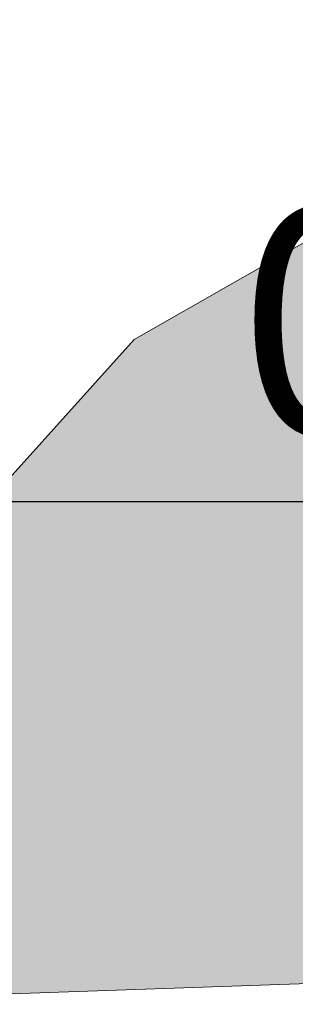
# Model space of a CAD drawing. Units: inches. Extents: x 2091 to 2899, y 967 to 2217.
# Tile 251 of 256: x 2217.01 to 2221.88, y 1131.25 to 1148.63. Entities that reach past the tile are written whole.
import ezdxf

# ---------------------------------------------------------------- set-up
doc = ezdxf.new("R2010")
doc.units = ezdxf.units.IN
doc.layers.add('A-ANNO-DIMS', color=2, linetype='Continuous', lineweight=18)
doc.layers.add('L-PLNT-TREE', color=94, linetype='Continuous', lineweight=13)
doc.layers.add('A-WALL-PATT', color=141, linetype='Continuous', lineweight=13, true_color=0xadddf7)
doc.layers.add('L-PLNT-PATT', color=114, linetype='Continuous', lineweight=13, true_color=0x139b48)
doc.styles.get("Standard").update_dxf_attribs({"font": 'arial.ttf'})
doc.dimstyles.new('ISO-25', dxfattribs={"dimtxt": 4, "dimasz": 4, "dimexe": 1.25, "dimexo": 0.625, "dimtad": 1, "dimdec": 0, "dimlunit": 3, "dimtxsty": 'Standard', "dimcen": 2.5, "dimadec": 0, "dimazin": 0, "dimtfac": 1, "dimtdec": 0, "dimtmove": 0, "dimatfit": 3, "dimfxl": 1, "dimarcsym": 0})

# ---------------------------------------------------------------- blocks, each defined once
blk = doc.blocks.new('*U25')
blk.add_lwpolyline([(-1139.42368, 1783.79628), (-1216.11644, 1685.47796), (-1117.5111, 1601.2033), (-1051.7759, 1643.3419), (-1126.09884, 1521.20092), (-1072.10606, 1527.49758), (-1079.90386, 1416.93646), (-1259.93906, 1179.83508), (-1479.05978, 1165.78888), (-1577.66258, 1109.60662), (-1742.00312, 927.01364), (-1676.26538, 814.64658), (-1270.89408, 828.69278), (-1194.20386, 772.51052), (-1007.95074, 856.78518), (-876.4778, 575.87134), (-821.70016, 575.87134), (-569.71184, 884.87504)])
blk = doc.blocks.new('*D37')
at = {"layer": 'A-ANNO-DIMS', "color": 0, "lineweight": -2, "transparency": 16777216}
for p, q in [((2203.116, 1151.622), (2203.116, 1138.874)), ((2212.276, 1151.622), (2212.276, 1138.874)), ((2199.116, 1140.124), (2195.116, 1140.124)), ((2203.116, 1140.124), (2212.276, 1140.124)), ((2216.276, 1140.124), (2245.908, 1140.124))]:
    blk.add_line(p, q, dxfattribs=at)
at = {"layer": 'A-ANNO-DIMS', "color": 0, "transparency": 16777216}
for points in [[(2199.116, 1140.79), (2199.116, 1139.457), (2203.116, 1140.124)], [(2216.276, 1140.79), (2216.276, 1139.457), (2212.276, 1140.124)]]:
    blk.add_solid(points, dxfattribs=at)
at = {"layer": 'Defpoints', "color": 0, "transparency": 16777216}
for p in [(2203.116, 1152.247), (2212.276, 1152.247), (2212.276, 1140.124)]:
    blk.add_point(p, dxfattribs=at)
at = {"layer": 'A-ANNO-DIMS', "color": 0, "transparency": 16777216, "insert": (2233.092, 1142.791), "char_height": 4, "attachment_point": 5}
blk.add_mtext('0\'-9" TYP.', dxfattribs=at)
blk = doc.blocks.new('*D71')
at = {"layer": 'A-ANNO-DIMS', "color": 0, "lineweight": -2, "transparency": 16777216}
for p, q in [((2212.144, 1351.294), (2212.144, 969.464)), ((2452.144, 1351.294), (2452.144, 969.464)), ((2216.144, 970.714), (2448.144, 970.714))]:
    blk.add_line(p, q, dxfattribs=at)
at = {"layer": 'A-ANNO-DIMS', "color": 0, "transparency": 16777216}
for points in [[(2216.144, 971.381), (2216.144, 970.048), (2212.144, 970.714)], [(2448.144, 971.381), (2448.144, 970.048), (2452.144, 970.714)]]:
    blk.add_solid(points, dxfattribs=at)
at = {"layer": 'Defpoints', "color": 0, "transparency": 16777216}
for p in [(2212.144, 1351.919), (2452.144, 1351.919), (2452.144, 970.714)]:
    blk.add_point(p, dxfattribs=at)
at = {"layer": 'A-ANNO-DIMS', "color": 0, "transparency": 16777216, "insert": (2332.144, 973.382), "char_height": 4, "attachment_point": 5}
blk.add_mtext('20\'-0"', dxfattribs=at)
blk = doc.blocks.new('*D75')
at = {"layer": 'A-ANNO-DIMS', "color": 0, "lineweight": -2, "transparency": 16777216}
for p, q in [((2212.144, 1274.794), (2212.144, 969.464)), ((2308.144, 1274.794), (2308.144, 969.464)), ((2216.144, 970.714), (2304.144, 970.714))]:
    blk.add_line(p, q, dxfattribs=at)
at = {"layer": 'A-ANNO-DIMS', "color": 0, "transparency": 16777216}
for points in [[(2216.144, 971.381), (2216.144, 970.048), (2212.144, 970.714)], [(2304.144, 971.381), (2304.144, 970.048), (2308.144, 970.714)]]:
    blk.add_solid(points, dxfattribs=at)
at = {"layer": 'Defpoints', "color": 0, "transparency": 16777216}
for p in [(2212.144, 1275.419), (2308.144, 1275.419), (2308.144, 970.714)]:
    blk.add_point(p, dxfattribs=at)
at = {"layer": 'A-ANNO-DIMS', "color": 0, "transparency": 16777216, "insert": (2260.144, 973.382), "char_height": 4, "attachment_point": 5}
blk.add_mtext('8\'-0"', dxfattribs=at)

msp = doc.modelspace()

# ---------------------------------------------------------------- hatches: boundary and pattern name
at = {"layer": 'A-WALL-PATT'}
h = msp.add_hatch(color=256, dxfattribs=at)
h.dxf.hatch_style = 1
h.paths.add_polyline_path([(2803.144, 2050.919), (2203.144, 2050.919), (2203.144, 1090.919), (2803.144, 1090.919)])
h.paths.add_polyline_path([(2635.799, 1147.54), (2674.524, 1147.54, 0.376086), (2678.53, 1152.88), (2678.53, 1159.556, 0.333335), (2674.524, 1163.562), (2674.524, 1163.562), (2674.524, 1192.934), (2635.806, 1192.934), (2597.088, 1192.934), (2597.088, 1163.562, 0.333335), (2593.082, 1159.556), (2593.082, 1152.88, 0.376086), (2597.088, 1147.54)], flags=0)
h.paths.add_polyline_path([(2436.01, 1278.241, 0.000483), (2435.953, 1278.215, -0.001328), (2435.936, 1278.112, -0.001711), (2436.116, 1278.041, 0.002185)], flags=0)
h.paths.add_polyline_path([(2794.144, 1143.419), (2794.144, 1347.419), (2543.37, 1347.419), (2543.37, 1351.919), (2794.144, 1351.919), (2794.144, 1392.714), (2793.947, 1392.714), (2793.947, 1473.537), (2794.144, 1473.537), (2794.144, 1531.919), (2650.144, 1531.919), (2650.144, 1536.419), (2794.144, 1536.419), (2794.144, 1692.419), (2609.376, 1692.419), (2609.376, 1644.419), (2604.876, 1644.419), (2604.876, 1744.919), (2609.376, 1744.919), (2609.376, 1696.919), (2794.144, 1696.919), (2794.144, 1780.919), (2609.644, 1780.919), (2493.876, 1780.919), (2493.876, 1785.419), (2609.644, 1785.419), (2794.144, 1785.419), (2794.144, 1847.939), (2793.951, 1847.939), (2793.951, 1928.762), (2794.144, 1928.762), (2794.144, 1941.419), (2614.144, 1941.419), (2614.144, 1821.419), (2609.644, 1821.419), (2609.644, 1941.419), (2392.144, 1941.419), (2392.144, 1819.919), (2387.644, 1819.919), (2387.644, 1941.419), (2212.144, 1941.419), (2212.144, 1783.919), (2392.144, 1783.919), (2392.144, 1780.919), (2212.144, 1780.919), (2212.144, 1629.419), (2387.644, 1629.419), (2387.644, 1744.919), (2392.144, 1744.919), (2392.144, 1627.919), (2317.144, 1627.919), (2317.144, 1551.419), (2317.144, 1536.419), (2459.384, 1536.419), (2459.384, 1602.396), (2463.884, 1602.396), (2463.884, 1531.919), (2456.644, 1531.919), (2456.644, 1529.919), (2452.144, 1529.919), (2452.144, 1531.919), (2312.644, 1531.919), (2312.644, 1551.419), (2306.144, 1551.419), (2306.144, 1555.919), (2308.144, 1555.919), (2308.144, 1551.419), (2312.644, 1551.419), (2312.644, 1627.919), (2212.144, 1627.919), (2212.144, 1555.919), (2270.144, 1555.919), (2270.144, 1551.419), (2212.144, 1551.419), (2212.144, 1351.919), (2272.144, 1351.919), (2272.144, 1347.419), (2212.144, 1347.419), (2212.144, 1275.419), (2308.144, 1275.419), (2308.144, 1351.919), (2452.144, 1351.919), (2452.144, 1493.919), (2456.644, 1493.919), (2456.644, 1347.419), (2312.644, 1347.419), (2312.644, 1270.919), (2212.144, 1270.919), (2212.144, 1099.919), (2281.238, 1099.919), (2282.871, 1110.914), (2282.008, 1116.997), (2278.558, 1121.42), (2268.206, 1128.056), (2272.088, 1128.056), (2273.813, 1131.927), (2279.42, 1134.692), (2285.028, 1135.245), (2287.616, 1137.457), (2288.047, 1138.01), (2289.341, 1140.775), (2291.067, 1139.669), (2292.361, 1135.245), (2295.38, 1136.904), (2296.243, 1135.798), (2297.105, 1133.033), (2300.125, 1138.01), (2303.144, 1138.01), (2304.438, 1135.798), (2303.144, 1133.586), (2306.595, 1134.692), (2307.889, 1133.033), (2310.908, 1135.245), (2313.927, 1134.139), (2315.627, 1132.427), (2308.32, 1117.55), (2290.204, 1109.808), (2288.91, 1103.172), (2289.272, 1099.919), (2434.918, 1099.919), (2431.593, 1124.788), (2429.93, 1169.553), (2430.927, 1240.52), (2435.659, 1238.186), (2437.135, 1196.554), (2438.798, 1143.973), (2442.678, 1111.998), (2446.558, 1099.919), (2794.144, 1099.919), (2794.144, 1138.919), (2548.032, 1138.919), (2548.032, 1143.419), (2548.032, 1148.819), (2546.668, 1148.032), (2528.686, 1179.179, 0.256256), (2512.032, 1148.819), (2512.032, 1143.419), (2512.032, 1138.919), (2507.532, 1138.919), (2507.532, 1143.419), (2507.532, 1148.819, 0.256256), (2490.879, 1179.179), (2472.896, 1148.032), (2471.532, 1148.819), (2471.532, 1143.419), (2467.032, 1143.419), (2467.032, 1269.946, 0.039061), (2460.91, 1273.58), (2467.032, 1273.58), (2467.032, 1286.325, 0.014511), (2465.216, 1286.762), (2467.032, 1287.053), (2467.032, 1323.419), (2471.532, 1323.419), (2471.532, 1148.819), (2489.532, 1179.996), (2490.896, 1179.208), (2490.879, 1179.179, -0.256256), (2507.532, 1148.819), (2507.532, 1143.419), (2512.032, 1143.419), (2512.032, 1148.819, -0.256256), (2528.686, 1179.179), (2528.668, 1179.208), (2530.032, 1179.996), (2548.032, 1148.819), (2548.032, 1143.419)], flags=16)
h.paths.add_polyline_path([(2607.769, 1200.945), (2607.769, 1265.031), (2597.088, 1281.052), (2619.785, 1281.052), (2627.795, 1337.127), (2635.799, 1337.127), (2643.817, 1337.127), (2651.827, 1281.052), (2674.524, 1281.052), (2663.843, 1265.031), (2663.843, 1200.945), (2635.806, 1200.945)], flags=0)
edge = h.paths.add_edge_path(flags=0)
edge.add_ellipse((13303.896, 1272.999), major_axis=(-10595.313, 0), ratio=0.84230387, start_angle=0.6282372, end_angle=0.6465541, ccw=False)
edge.add_ellipse((2711.7, 1156.853), major_axis=(2.22, 0), ratio=0.842304, start_angle=111.5352, end_angle=180.6282, ccw=False)
edge.add_ellipse((13303.156, 1272.999), major_axis=(-10593.026, 0), ratio=0.84230387, start_angle=0.5282715, end_angle=0.6465541, ccw=False)
edge.add_line((2710.765, 1175.333), (2710.13, 1175.333))
edge.add_ellipse((2710.13, 1176.58), major_axis=(1.48, 0), ratio=0.842304, start_angle=180, end_angle=270, ccw=False)
edge.add_line((2708.65, 1176.58), (2708.65, 1200.783))
edge.add_ellipse((2710.13, 1200.783), major_axis=(1.48, 0), ratio=0.842304, start_angle=90, end_angle=180, ccw=False)
edge.add_line((2710.13, 1202.029), (2710.465, 1202.029))
edge.add_ellipse((13303.156, 1272.999), major_axis=(-10593.026, 0), ratio=0.84230387, start_angle=-0.0902291, end_angle=0.3838668, ccw=False)
edge.add_ellipse((2710.13, 1290.927), major_axis=(-1.48, 0), ratio=0.842304, start_angle=0, end_angle=90, ccw=False)
edge.add_line((2708.65, 1290.927), (2708.65, 1315.13))
edge.add_ellipse((2710.13, 1315.13), major_axis=(-1.48, 0), ratio=0.842304, start_angle=-90, end_angle=0, ccw=False)
edge.add_line((2710.13, 1316.377), (2710.706, 1316.377))
edge.add_ellipse((3238.402, 1296.29), major_axis=(528.234, 0), ratio=0.8423039, start_angle=176.34957, end_angle=177.82005, ccw=False)
edge.add_ellipse((2775.063, 1071.451), major_axis=(313.308, 0), ratio=0.8423039, start_angle=102.12597, end_angle=103.78053, ccw=False)
edge.add_ellipse((2775.063, 1078.306), major_axis=(-305.303, 0), ratio=0.8423039, start_angle=-79.79046, end_angle=-77.55537, ccw=False)
edge.add_ellipse((2695.142, 1541.975), major_axis=(-250.96, 0), ratio=0.8423039, start_angle=99.25657, end_angle=102.55493)
edge.add_line((2741.41, 1334.214), (2747.133, 1337.378))
edge.add_ellipse((2747.539, 1336.857), major_axis=(-0.74, 0), ratio=0.842304, start_angle=270, end_angle=307.9331, ccw=False)
edge.add_ellipse((2747.539, 1336.857), major_axis=(-0.74, 0), ratio=0.842304, start_angle=232.0669, end_angle=270, ccw=False)
edge.add_line((2747.945, 1337.378), (2753.667, 1334.214))
edge.add_ellipse((2799.935, 1541.975), major_axis=(250.96, 0), ratio=0.8423039, start_angle=257.44507, end_angle=260.74343)
edge.add_ellipse((2720.014, 1078.306), major_axis=(305.303, 0), ratio=0.8423039, start_angle=77.55537, end_angle=79.79046, ccw=False)
edge.add_ellipse((2720.014, 1071.451), major_axis=(-313.308, 0), ratio=0.8423039, start_angle=256.21947, end_angle=257.87403, ccw=False)
edge.add_ellipse((2256.676, 1296.29), major_axis=(-528.234, 0), ratio=0.8423039, start_angle=182.17995, end_angle=183.65043, ccw=False)
edge.add_line((2784.371, 1316.377), (2784.947, 1316.377))
edge.add_ellipse((2784.947, 1315.13), major_axis=(1.48, 0), ratio=0.842304, start_angle=0, end_angle=90, ccw=False)
edge.add_line((2786.427, 1315.13), (2786.427, 1290.927))
edge.add_ellipse((2784.947, 1290.927), major_axis=(1.48, 0), ratio=0.842304, start_angle=270, end_angle=360, ccw=False)
edge.add_ellipse((-7808.079, 1272.999), major_axis=(10593.026, 0), ratio=0.84230387, start_angle=-0.3838668, end_angle=0.0902291, ccw=False)
edge.add_line((2784.612, 1202.029), (2784.947, 1202.029))
edge.add_ellipse((2784.947, 1200.783), major_axis=(1.48, 0), ratio=0.842304, start_angle=0, end_angle=90, ccw=False)
edge.add_line((2786.427, 1200.783), (2786.427, 1176.58))
edge.add_ellipse((2784.947, 1176.58), major_axis=(-1.48, 0), ratio=0.842304, start_angle=90, end_angle=180, ccw=False)
edge.add_line((2784.947, 1175.333), (2784.313, 1175.333))
edge.add_ellipse((-7808.079, 1272.999), major_axis=(10593.026, 0), ratio=0.84230387, start_angle=-0.6186432, end_angle=-0.5282715, ccw=False)
edge.add_ellipse((2783.377, 1156.853), major_axis=(-2.22, 0), ratio=0.842304, start_angle=179.3718, end_angle=248.4648, ccw=False)
edge.add_ellipse((-7808.819, 1272.999), major_axis=(-10595.313, 0), ratio=0.842303866, start_angle=179.3534459, end_angle=179.3717628, ccw=False)
edge.add_ellipse((2780.297, 1153.501), major_axis=(-5.246, 0), ratio=0.842304, start_angle=90, end_angle=179.3534, ccw=False)
edge.add_line((2780.297, 1149.082), (2714.78, 1149.082))
edge.add_ellipse((2714.78, 1153.501), major_axis=(5.246, 0), ratio=0.842304, start_angle=180.6466, end_angle=270, ccw=False)
edge = h.paths.add_edge_path(flags=0)
edge.add_line((2718.187, 1151.008), (2718.187, 1170.472))
edge.add_ellipse((2721.147, 1170.472), major_axis=(-2.96, 0), ratio=0.842304, start_angle=-90, end_angle=0, ccw=False)
edge.add_line((2721.147, 1172.965), (2773.93, 1172.965))
edge.add_ellipse((2773.93, 1170.472), major_axis=(-2.96, 0), ratio=0.842304, start_angle=180, end_angle=270, ccw=False)
edge.add_line((2776.89, 1170.472), (2776.89, 1151.008))
edge.add_line((2776.89, 1151.008), (2718.187, 1151.008))
edge = h.paths.add_edge_path(flags=0)
edge.add_line((2718.187, 1180.234), (2718.187, 1199.058))
edge.add_ellipse((2747.539, 1320.399), major_axis=(147.018, 0), ratio=0.8423039, start_angle=256.40187, end_angle=283.59813)
edge.add_line((2776.89, 1199.058), (2776.89, 1180.234))
edge.add_ellipse((2747.539, 1301.575), major_axis=(147.018, 0), ratio=0.8423039, start_angle=256.40187, end_angle=283.59813, ccw=False)
edge = h.paths.add_edge_path(flags=0)
edge.add_ellipse((13303.156, 1272.999), major_axis=(-10591.546, 0), ratio=0.84230387, start_angle=0.0555943, end_angle=0.3777642, ccw=False)
edge.add_line((2711.617, 1262.722), (2715.667, 1249.495))
edge.add_ellipse((6413.892, 1241.692), major_axis=(-3698.236, 0), ratio=0.84230387, start_angle=-0.120897, end_angle=0.364076)
edge.add_line((2715.761, 1218.192), (2711.934, 1203.167))
edge = h.paths.add_edge_path(flags=0)
edge.add_line((2718.187, 1251.075), (2716.002, 1267.45))
edge.add_ellipse((2742.151, 1202.19), major_axis=(81.773, 0), ratio=0.842304, start_angle=94.27742, end_angle=111.83495, ccw=False)
edge.add_line((2737.01, 1270.931), (2758.067, 1270.931))
edge.add_ellipse((2752.926, 1202.19), major_axis=(81.773, 0), ratio=0.842304, start_angle=68.16505, end_angle=85.72258, ccw=False)
edge.add_line((2779.075, 1267.45), (2776.89, 1251.075))
edge.add_ellipse((2750.338, 1187.885), major_axis=(79.58, 0), ratio=0.842304, start_angle=67.20809, end_angle=85.12993)
edge.add_line((2756.035, 1254.744), (2739.043, 1254.744))
edge.add_ellipse((2744.739, 1187.885), major_axis=(79.58, 0), ratio=0.842304, start_angle=94.87007, end_angle=112.79191)
edge = h.paths.add_edge_path(flags=0)
edge.add_line((2783.143, 1203.167), (2779.316, 1218.192))
edge.add_ellipse((-918.815, 1241.692), major_axis=(3698.236, 0), ratio=0.84230387, start_angle=-0.364076, end_angle=0.120897)
edge.add_line((2779.41, 1249.495), (2783.46, 1262.722))
edge.add_ellipse((-7808.079, 1272.999), major_axis=(-10591.546, 0), ratio=0.84230387, start_angle=179.6222358, end_angle=179.9444057, ccw=False)
edge = h.paths.add_edge_path(flags=0)
edge.add_ellipse((2734.201, 1286.69), major_axis=(-0.357, 6.34), ratio=0.603834, start_angle=89.002, end_angle=253.6574, ccw=False)
edge.add_line((2730.369, 1286.542), (2730.369, 1301.352))
edge.add_line((2730.369, 1301.352), (2735.913, 1305.215))
edge.add_ellipse((2736.385, 1304.735), major_axis=(0.74, 0), ratio=0.842304, start_angle=90, end_angle=134.4802, ccw=False)
edge.add_line((2736.385, 1305.358), (2738.033, 1305.358))
edge.add_line((2738.033, 1305.358), (2738.033, 1307.708))
edge.add_ellipse((2794.202, 1307.708), major_axis=(56.169, 0), ratio=0.842304, start_angle=150.5614, end_angle=180, ccw=False)
edge.add_ellipse((2700.876, 1307.708), major_axis=(-56.169, 0), ratio=0.842304, start_angle=180, end_angle=209.4386, ccw=False)
edge.add_line((2757.044, 1307.708), (2757.044, 1305.358))
edge.add_line((2757.044, 1305.358), (2758.692, 1305.358))
edge.add_ellipse((2758.692, 1304.735), major_axis=(-0.74, 0), ratio=0.842304, start_angle=225.5198, end_angle=270, ccw=False)
edge.add_line((2759.164, 1305.215), (2764.708, 1301.352))
edge.add_line((2764.708, 1301.352), (2764.708, 1286.542))
edge.add_ellipse((2760.876, 1286.69), major_axis=(0.357, 6.34), ratio=0.603834, start_angle=106.3426, end_angle=270.998, ccw=False)
edge.add_line((2757.044, 1285.797), (2757.044, 1307.708))
edge.add_ellipse((2700.876, 1307.708), major_axis=(-56.169, 0), ratio=0.842304, start_angle=180, end_angle=209.4386)
edge.add_ellipse((2794.202, 1307.708), major_axis=(56.169, 0), ratio=0.842304, start_angle=150.5614, end_angle=180)
edge.add_line((2738.033, 1307.708), (2738.033, 1285.797))
h.paths.add_polyline_path([(2417.812, 1104.45), (2413.492, 1102.53), (2410.612, 1103.97), (2409.172, 1106.37), (2407.252, 1107.33), (2406.292, 1109.73), (2405.332, 1114.05), (2405.332, 1117.89), (2406.292, 1120.13), (2407.252, 1119.81), (2408.848, 1118.328), (2410.174, 1119.424), (2410.211, 1120.406), (2411.041, 1121.419), (2410.699, 1119.859), (2410.174, 1119.424), (2410.088, 1117.176), (2411.133, 1116.206), (2413.972, 1119.33), (2416.852, 1120.77), (2416.87, 1120.799), (2417.035, 1119.405), (2417.896, 1118.143), (2418.292, 1118.37), (2419.544, 1120.039), (2419.361, 1118.387), (2419.032, 1119.356), (2418.399, 1118.512), (2419.252, 1114.53), (2418.794, 1107.199)], flags=0)
h.paths.add_polyline_path([(2508.87, 1347.419), (2508.37, 1347.419), (2508.37, 1351.919), (2508.87, 1351.919)], flags=0)
h.paths.add_polyline_path([(2473.37, 1347.419), (2472.37, 1347.419), (2467.87, 1347.419), (2467.87, 1455.419), (2472.37, 1455.419), (2472.37, 1352.419), (2473.37, 1352.419)], flags=0)
h.paths.add_polyline_path([(2352.106, 1217.446), (2349.226, 1218.886), (2347.786, 1221.286), (2345.866, 1222.246), (2344.906, 1224.646), (2343.946, 1228.966), (2343.946, 1232.806), (2344.906, 1235.046), (2345.866, 1234.726), (2347.462, 1233.244), (2348.788, 1234.341), (2348.825, 1235.322), (2349.655, 1236.336), (2349.313, 1234.775), (2348.788, 1234.341), (2348.702, 1232.093), (2349.747, 1231.123), (2352.586, 1234.246), (2355.466, 1235.686), (2355.484, 1235.715), (2355.649, 1234.322), (2356.51, 1233.06), (2356.906, 1233.286), (2358.158, 1234.956), (2357.975, 1233.304), (2357.646, 1234.273), (2357.013, 1233.428), (2357.866, 1229.446), (2357.408, 1222.115), (2356.426, 1219.366)], flags=0)
h.paths.add_polyline_path([(2348.297, 1112.224), (2347.014, 1112.31), (2345.53, 1114.127), (2345.732, 1115.858), (2346.812, 1116.982), (2346.812, 1114.646), (2345.867, 1114.214), (2346.88, 1114.3)], flags=0)
h.paths.add_polyline_path([(2347.014, 1110.926), (2346.272, 1110.493), (2346.61, 1111.186)], flags=0)
h.paths.add_polyline_path([(2345.867, 1118.194), (2345.53, 1117.329), (2343.708, 1118.021), (2344.383, 1118.626)], flags=0)
h.paths.add_polyline_path([(2346.677, 1109.282), (2346.07, 1108.071), (2345.867, 1110.061)], flags=0)
h.paths.add_polyline_path([(2345.057, 1119.751), (2343.64, 1119.751), (2343.978, 1121.135)], flags=0)
h.paths.add_polyline_path([(2345.26, 1116.55), (2345.125, 1115.858), (2344.922, 1115.685), (2344.72, 1116.377)], flags=0)
h.paths.add_polyline_path([(2345.665, 1112.31), (2345.462, 1111.532), (2344.045, 1111.964), (2344.652, 1112.57)], flags=0)
h.paths.add_polyline_path([(2345.192, 1113.349), (2344.45, 1113.868), (2344.72, 1114.387)], flags=0)
h.paths.add_polyline_path([(2344.652, 1116.809), (2344.18, 1115.685), (2344.652, 1115.339), (2343.91, 1114.906), (2343.033, 1115.944), (2343.64, 1116.463)], flags=0)
h.paths.add_polyline_path([(2345.867, 1106.686), (2344.99, 1105.562), (2344.517, 1106.6)], flags=0)
h.paths.add_polyline_path([(2344.855, 1110.061), (2344.517, 1109.282), (2344.113, 1109.715)], flags=0)
h.paths.add_polyline_path([(2344.045, 1113.522), (2343.438, 1113.089), (2342.763, 1113.954)], flags=0)
h.paths.add_polyline_path([(2344.315, 1111.012), (2342.965, 1110.32), (2342.965, 1111.099)], flags=0)
h.paths.add_polyline_path([(2345.125, 1104.697), (2344.585, 1103.745), (2344.45, 1104.264)], flags=0)
h.paths.add_polyline_path([(2342.83, 1121.222), (2341.75, 1120.53), (2340.536, 1121.049), (2340.131, 1121.828), (2340.671, 1122.952), (2341.143, 1121.828), (2341.615, 1122.001)], flags=0)
h.paths.add_polyline_path([(2342.965, 1119.751), (2343.033, 1118.453), (2342.088, 1118.021), (2342.02, 1119.491)], flags=0)
h.paths.add_polyline_path([(2342.695, 1116.896), (2341.953, 1116.636), (2342.02, 1117.329)], flags=0)
h.paths.add_polyline_path([(2343.033, 1112.224), (2342.02, 1111.791), (2341.548, 1112.224), (2342.358, 1113.349)], flags=0)
h.paths.add_polyline_path([(2343.775, 1104.437), (2342.628, 1102.88), (2342.695, 1104.61), (2343.438, 1105.129)], flags=0)
h.paths.add_polyline_path([(2342.02, 1115.079), (2340.806, 1115.512), (2340.941, 1116.377)], flags=0)
h.paths.add_polyline_path([(2341.481, 1120.097), (2341.481, 1119.405), (2341.076, 1119.578), (2341.143, 1120.097)], flags=0)
h.paths.add_polyline_path([(2341.818, 1114.473), (2340.941, 1113.089), (2340.806, 1114.56)], flags=0)
h.paths.add_polyline_path([(2341.143, 1118.54), (2340.941, 1116.982), (2339.051, 1117.675), (2339.051, 1118.626)], flags=0)
h.paths.add_polyline_path([(2342.695, 1101.668), (2341.953, 1101.841), (2342.56, 1102.361)], flags=0)
h.paths.add_polyline_path([(2340.333, 1119.665), (2338.444, 1119.578), (2337.904, 1120.357), (2339.658, 1120.616)], flags=0)
h.paths.add_polyline_path([(2340.333, 1115.339), (2340.063, 1113.695), (2339.388, 1115.339)], flags=0)
h.paths.add_polyline_path([(2341.818, 1103.831), (2341.548, 1102.88), (2341.143, 1103.658)], flags=0)
h.paths.add_polyline_path([(2339.051, 1122.866), (2337.296, 1121.828), (2337.094, 1123.125), (2337.769, 1123.818)], flags=0)
h.paths.add_polyline_path([(2339.118, 1121.741), (2338.848, 1121.222), (2338.174, 1121.049), (2338.376, 1121.568)], flags=0)
h.paths.add_polyline_path([(2339.186, 1119.319), (2338.646, 1118.713), (2338.241, 1118.107), (2338.241, 1118.886)], flags=0)
h.paths.add_polyline_path([(2341.143, 1101.928), (2340.603, 1101.236), (2340.063, 1101.841), (2340.603, 1102.361)], flags=0)
h.paths.add_polyline_path([(2337.634, 1117.761), (2336.621, 1118.28), (2337.296, 1118.972)], flags=0)
h.paths.add_polyline_path([(2336.824, 1119.578), (2334.799, 1118.972), (2335.204, 1120.357), (2336.554, 1120.876)], flags=0)
h.paths.add_polyline_path([(2339.118, 1100.457), (2337.364, 1100.543), (2336.756, 1101.236)], flags=0)
h.paths.add_polyline_path([(2336.351, 1122.433), (2336.014, 1121.914), (2334.934, 1122.433), (2334.529, 1123.471), (2335.744, 1122.779)], flags=0)
h.paths.add_polyline_path([(2334.732, 1120.876), (2334.259, 1120.357), (2334.057, 1120.789), (2334.597, 1121.308)], flags=0)
h.paths.add_polyline_path([(2334.462, 1122.174), (2332.572, 1121.308), (2331.357, 1122.174), (2332.1, 1122.866)], flags=0)
h.paths.add_polyline_path([(2334.259, 1118.54), (2333.382, 1118.453), (2333.652, 1119.319)], flags=0)
h.paths.add_polyline_path([(2335.542, 1102.274), (2334.192, 1102.62), (2335.272, 1103.312)], flags=0)
h.paths.add_polyline_path([(2332.707, 1119.665), (2331.695, 1120.443), (2332.505, 1120.789)], flags=0)
h.paths.add_polyline_path([(2334.732, 1101.149), (2333.517, 1101.582), (2333.989, 1101.755)], flags=0)
h.paths.add_polyline_path([(2332.64, 1116.636), (2331.087, 1116.29), (2331.965, 1118.194)], flags=0)
h.paths.add_polyline_path([(2330.75, 1121.568), (2330.277, 1120.27), (2328.523, 1119.319), (2328.995, 1121.049)], flags=0)
h.paths.add_polyline_path([(2330.75, 1118.626), (2330.008, 1117.502), (2329.873, 1118.021)], flags=0)
h.paths.add_polyline_path([(2332.1, 1102.361), (2330.547, 1102.014), (2331.695, 1102.966)], flags=0)
h.paths.add_polyline_path([(2329.535, 1113.608), (2329.063, 1112.31), (2328.59, 1113.349)], flags=0)
h.paths.add_polyline_path([(2328.388, 1117.848), (2327.51, 1116.55), (2327.173, 1117.761)], flags=0)
h.paths.add_polyline_path([(2329.738, 1106.513), (2329.535, 1105.302), (2328.253, 1106.081)], flags=0)
h.paths.add_polyline_path([(2328.658, 1114.387), (2328.05, 1114.127), (2328.32, 1114.906)], flags=0)
h.paths.add_polyline_path([(2328.32, 1112.224), (2327.106, 1112.137), (2326.701, 1112.656)], flags=0)
h.paths.add_polyline_path([(2326.903, 1115.252), (2326.701, 1114.127), (2325.216, 1113.608), (2326.093, 1115.339)], flags=0)
h.paths.add_polyline_path([(2326.633, 1108.33), (2326.093, 1107.379), (2325.891, 1108.503), (2326.498, 1109.109)], flags=0)
h.paths.add_polyline_path([(2615.144, 1531.919), (2609.644, 1531.919), (2609.644, 1620.419), (2614.144, 1620.419), (2614.144, 1536.419), (2615.144, 1536.419)], flags=0)
h.paths.add_polyline_path([(2545.144, 1563.419), (2464.144, 1563.419), (2464.144, 1632.419), (2509.144, 1632.419), (2509.144, 1627.919), (2509.144, 1603.919), (2468.644, 1603.919), (2468.644, 1567.919), (2540.644, 1567.919), (2540.644, 1591.919), (2545.144, 1591.919)], flags=0)
h.paths.add_polyline_path([(2388.969, 1549.986), (2357.434, 1549.986), (2357.434, 1623.361), (2399.363, 1623.361), (2435.689, 1623.361), (2435.593, 1602.559), (2435.593, 1602.396), (2388.969, 1602.396)], flags=0)
h.paths.add_polyline_path([(2388.881, 1555.809), (2374.904, 1555.809), (2374.904, 1600.572), (2374.904, 1615.458), (2406.351, 1615.458), (2406.351, 1618.939), (2412.174, 1615.458), (2406.351, 1611.976), (2406.351, 1615.458), (2388.881, 1615.458)], flags=0)
h.paths.add_polyline_path([(2568.876, 1644.419), (2453.376, 1644.419), (2453.376, 1785.419), (2457.876, 1785.419), (2457.876, 1648.919), (2568.876, 1648.919)], flags=0)
h.paths.add_polyline_path([(2212.144, 1945.919), (2212.144, 2041.919), (2794.144, 2041.919), (2794.144, 1945.919)], flags=16)
h.paths.add_polyline_path([(2271.083, 1964.317), (2776.853, 1964.317), (2776.853, 2037.17), (2271.083, 2037.17)], flags=8)
h.paths.add_polyline_path([(2380.649, 1536.824), (2461.041, 1536.824), (2461.041, 1554.653), (2380.649, 1554.653)], flags=8)
h.paths.add_polyline_path([(2240.756, 1609.725), (2309.186, 1609.725), (2309.186, 1617.698), (2240.756, 1617.698)], flags=8)
h.paths.add_polyline_path([(2212.677, 1313.504), (2282.592, 1313.504), (2282.592, 1322.745), (2212.677, 1322.745)], flags=8)
h.paths.add_polyline_path([(2457.112, 1114.779), (2558.482, 1114.779), (2558.482, 1142.22), (2457.112, 1142.22)], flags=8)
h.paths.add_polyline_path([(2473.442, 1273.01), (2604.641, 1273.01), (2604.641, 1318.347), (2473.442, 1318.347)], flags=8)
h.paths.add_polyline_path([(2638.876, 1626.977), (2684.25, 1627.977), (2684.038, 1637.597), (2638.664, 1636.598)], flags=8)
h.paths.add_polyline_path([(2537.591, 1453.793), (2628.39, 1453.793), (2628.39, 1475.345), (2537.591, 1475.345)], flags=8)
h.paths.add_polyline_path([(2504.138, 1714.632), (2554.647, 1714.632), (2554.647, 1730.238), (2504.138, 1730.238)], flags=8)
h.paths.add_polyline_path([(2487.501, 1575.652), (2535.097, 1575.652), (2535.097, 1598.378), (2487.501, 1598.378)], flags=8)
h.paths.add_polyline_path([(2709.099, 1735.71), (2740.017, 1735.71), (2740.017, 1749.938), (2709.099, 1749.938)], flags=8)
h.paths.add_polyline_path([(2442.438, 1792.172), (2564.729, 1792.172), (2564.729, 1842), (2442.438, 1842)], flags=8)
h.paths.add_polyline_path([(2655.816, 1809.644), (2789.52, 1806.694), (2790.085, 1832.292), (2656.381, 1835.242)], flags=8)
h.paths.add_polyline_path([(2234.843, 1797.72), (2368.593, 1794.769), (2369.161, 1820.504), (2235.411, 1823.455)], flags=8)
h.paths.add_polyline_path([(2245.138, 1644.006), (2398.428, 1640.624), (2398.995, 1666.325), (2245.706, 1669.707)], flags=8)
h.paths.add_polyline_path([(2306.143, 1431.169), (2413.768, 1428.794), (2414.333, 1454.392), (2306.708, 1456.766)], flags=8)
h.paths.add_polyline_path([(2306.835, 1458.233), (2393.38, 1456.323), (2393.933, 1481.354), (2307.387, 1483.264)], flags=8)
at = {"layer": 'L-PLNT-PATT'}
h = msp.add_hatch(color=256, dxfattribs=at)
h.dxf.hatch_style = 1
h.paths.add_polyline_path([(2333.338, 1165.659), (2329.024, 1166.212), (2331.612, 1168.424), (2335.063, 1177.271), (2328.162, 1184.46), (2319.535, 1187.225), (2323.417, 1193.308), (2319.966, 1203.814), (2317.809, 1203.814), (2313.496, 1213.215), (2310.908, 1212.662), (2307.889, 1212.662), (2305.732, 1217.086), (2307.026, 1223.168), (2310.477, 1223.168), (2304.007, 1230.91), (2303.136, 1237.046), (2299.693, 1240.864), (2296.674, 1237.546), (2294.949, 1238.652), (2294.517, 1241.417), (2292.361, 1242.523), (2289.341, 1239.758), (2285.89, 1240.311), (2283.302, 1235.334), (2283.302, 1230.91), (2286.753, 1229.251), (2284.165, 1227.592), (2281.577, 1229.804), (2274.244, 1222.615), (2274.244, 1220.957), (2271.225, 1219.298), (2272.088, 1217.639), (2274.244, 1214.321), (2270.362, 1211.556), (2266.48, 1214.321), (2264.324, 1213.768), (2263.461, 1211.556), (2266.48, 1211.003), (2266.912, 1206.579), (2263.539, 1207.132), (2259.579, 1203.261), (2263.892, 1202.708), (2262.167, 1197.178), (2258.285, 1196.625), (2253.971, 1193.861), (2248.795, 1191.096), (2248.364, 1193.308), (2244.482, 1185.013), (2251.383, 1186.672), (2255.697, 1183.907), (2254.403, 1177.271), (2246.639, 1174.506), (2243.188, 1176.718), (2241.894, 1173.4), (2238.875, 1172.847), (2236.287, 1169.53), (2233.267, 1165.659), (2237.149, 1162.341), (2239.737, 1164), (2236.811, 1159.191), (2238.937, 1159.439), (2238.63, 1155.086), (2231.542, 1145.752), (2222.915, 1145.199), (2219.033, 1142.987), (2212.563, 1135.798), (2215.151, 1131.374), (2231.111, 1131.927), (2234.13, 1129.715), (2241.463, 1133.033), (2246.639, 1121.973), (2248.795, 1121.973), (2258.716, 1134.139), (2261.736, 1135.798), (2263.892, 1133.033), (2263.892, 1129.162), (2267.343, 1128.056), (2272.088, 1128.056), (2273.813, 1131.927), (2279.42, 1134.692), (2285.028, 1135.245), (2287.616, 1137.457), (2288.047, 1138.01), (2289.341, 1140.775), (2291.067, 1139.669), (2292.361, 1135.245), (2295.38, 1136.904), (2296.243, 1135.798), (2297.105, 1133.033), (2300.125, 1138.01), (2303.144, 1138.01), (2304.438, 1135.798), (2303.144, 1133.586), (2306.595, 1134.692), (2307.889, 1133.033), (2310.908, 1135.245), (2313.927, 1134.139), (2319.966, 1128.056), (2322.554, 1126.95), (2324.711, 1124.738), (2342.827, 1126.397), (2346.278, 1123.079), (2348.866, 1124.185), (2341.964, 1133.033), (2341.533, 1136.351), (2343.69, 1139.669), (2339.808, 1150.175), (2337.651, 1150.175)])
h.paths.add_polyline_path([(2339.658, 1120.616), (2337.904, 1120.357), (2338.444, 1119.578), (2340.333, 1119.665)])
h.paths.add_polyline_path([(2341.143, 1118.54), (2339.051, 1118.626), (2339.051, 1117.675), (2340.941, 1116.982)])
h.paths.add_polyline_path([(2336.554, 1120.876), (2335.204, 1120.357), (2334.799, 1118.972), (2336.824, 1119.578)])
h.paths.add_polyline_path([(2337.296, 1118.972), (2336.621, 1118.28), (2337.634, 1117.761)])
h.paths.add_polyline_path([(2338.646, 1118.713), (2339.186, 1119.319), (2338.241, 1118.886), (2338.241, 1118.107)])
h.paths.add_polyline_path([(2339.051, 1122.866), (2337.769, 1123.818), (2337.094, 1123.125), (2337.296, 1121.828)])
h.paths.add_polyline_path([(2341.615, 1122.001), (2341.143, 1121.828), (2340.671, 1122.952), (2340.131, 1121.828), (2340.536, 1121.049), (2341.75, 1120.53), (2342.83, 1121.222)])
h.paths.add_polyline_path([(2342.965, 1119.751), (2342.02, 1119.491), (2342.088, 1118.021), (2343.033, 1118.453)])
h.paths.add_polyline_path([(2345.867, 1118.194), (2344.383, 1118.626), (2343.708, 1118.021), (2345.53, 1117.329)])
h.paths.add_polyline_path([(2344.652, 1116.809), (2343.64, 1116.463), (2343.033, 1115.944), (2343.91, 1114.906), (2344.652, 1115.339), (2344.18, 1115.685)])
h.paths.add_polyline_path([(2346.812, 1116.982), (2345.732, 1115.858), (2345.53, 1114.127), (2347.014, 1112.31), (2348.297, 1112.224), (2346.88, 1114.3), (2345.867, 1114.214), (2346.812, 1114.646)])
h.paths.add_polyline_path([(2345.26, 1116.55), (2344.72, 1116.377), (2344.922, 1115.685), (2345.125, 1115.858)])
h.paths.add_polyline_path([(2342.695, 1116.896), (2342.02, 1117.329), (2341.953, 1116.636)])
h.paths.add_polyline_path([(2341.481, 1120.097), (2341.143, 1120.097), (2341.076, 1119.578), (2341.481, 1119.405)])
h.paths.add_polyline_path([(2343.978, 1121.135), (2343.64, 1119.751), (2345.057, 1119.751)])
h.paths.add_polyline_path([(2339.118, 1121.741), (2338.376, 1121.568), (2338.174, 1121.049), (2338.848, 1121.222)])
h.paths.add_polyline_path([(2336.351, 1122.433), (2335.744, 1122.779), (2334.529, 1123.471), (2334.934, 1122.433), (2336.014, 1121.914)])
h.paths.add_polyline_path([(2334.462, 1122.174), (2332.1, 1122.866), (2331.357, 1122.174), (2332.572, 1121.308)])
h.paths.add_polyline_path([(2334.597, 1121.308), (2334.057, 1120.789), (2334.259, 1120.357), (2334.732, 1120.876)])
h.paths.add_polyline_path([(2332.505, 1120.789), (2331.695, 1120.443), (2332.707, 1119.665)])
h.paths.add_polyline_path([(2333.652, 1119.319), (2333.382, 1118.453), (2334.259, 1118.54)])
h.paths.add_polyline_path([(2331.965, 1118.194), (2331.087, 1116.29), (2332.64, 1116.636)])
h.paths.add_polyline_path([(2330.75, 1121.568), (2328.995, 1121.049), (2328.523, 1119.319), (2330.277, 1120.27)])
h.paths.add_polyline_path([(2330.75, 1118.626), (2329.873, 1118.021), (2330.008, 1117.502)])
h.paths.add_polyline_path([(2328.388, 1117.848), (2327.173, 1117.761), (2327.51, 1116.55)])
h.paths.add_polyline_path([(2326.903, 1115.252), (2326.093, 1115.339), (2325.216, 1113.608), (2326.701, 1114.127)])
h.paths.add_polyline_path([(2328.658, 1114.387), (2328.32, 1114.906), (2328.05, 1114.127)])
h.paths.add_polyline_path([(2326.701, 1112.656), (2327.106, 1112.137), (2328.32, 1112.224)])
h.paths.add_polyline_path([(2329.535, 1113.608), (2328.59, 1113.349), (2329.063, 1112.31)])
h.paths.add_polyline_path([(2340.333, 1115.339), (2339.388, 1115.339), (2340.063, 1113.695)])
h.paths.add_polyline_path([(2340.941, 1116.377), (2340.806, 1115.512), (2342.02, 1115.079)])
h.paths.add_polyline_path([(2341.818, 1114.473), (2340.806, 1114.56), (2340.941, 1113.089)])
h.paths.add_polyline_path([(2343.033, 1112.224), (2342.358, 1113.349), (2341.548, 1112.224), (2342.02, 1111.791)])
h.paths.add_polyline_path([(2342.763, 1113.954), (2343.438, 1113.089), (2344.045, 1113.522)])
h.paths.add_polyline_path([(2344.72, 1114.387), (2344.45, 1113.868), (2345.192, 1113.349)])
h.paths.add_polyline_path([(2345.665, 1112.31), (2344.652, 1112.57), (2344.045, 1111.964), (2345.462, 1111.532)])
h.paths.add_polyline_path([(2344.315, 1111.012), (2342.965, 1111.099), (2342.965, 1110.32)])
h.paths.add_polyline_path([(2344.855, 1110.061), (2344.113, 1109.715), (2344.517, 1109.282)])
h.paths.add_polyline_path([(2346.677, 1109.282), (2345.867, 1110.061), (2346.07, 1108.071)])
h.paths.add_polyline_path([(2347.014, 1110.926), (2346.61, 1111.186), (2346.272, 1110.493)])
h.paths.add_polyline_path([(2345.867, 1106.686), (2344.517, 1106.6), (2344.99, 1105.562)])
h.paths.add_polyline_path([(2345.125, 1104.697), (2344.45, 1104.264), (2344.585, 1103.745)])
h.paths.add_polyline_path([(2343.775, 1104.437), (2343.438, 1105.129), (2342.695, 1104.61), (2342.628, 1102.88)])
h.paths.add_polyline_path([(2341.818, 1103.831), (2341.143, 1103.658), (2341.548, 1102.88)])
h.paths.add_polyline_path([(2342.56, 1102.361), (2341.953, 1101.841), (2342.695, 1101.668)])
h.paths.add_polyline_path([(2341.143, 1101.928), (2340.603, 1102.361), (2340.063, 1101.841), (2340.603, 1101.236)])
h.paths.add_polyline_path([(2336.756, 1101.236), (2337.364, 1100.543), (2339.118, 1100.457)])
h.paths.add_polyline_path([(2335.272, 1103.312), (2334.192, 1102.62), (2335.542, 1102.274)])
h.paths.add_polyline_path([(2333.989, 1101.755), (2333.517, 1101.582), (2334.732, 1101.149)])
h.paths.add_polyline_path([(2331.695, 1102.966), (2330.547, 1102.014), (2332.1, 1102.361)])
h.paths.add_polyline_path([(2329.738, 1106.513), (2328.253, 1106.081), (2329.535, 1105.302)])
h.paths.add_polyline_path([(2326.633, 1108.33), (2326.498, 1109.109), (2325.891, 1108.503), (2326.093, 1107.379)])
h.paths.add_polyline_path([(2240.596, 1257.814), (2239.584, 1257.468), (2238.977, 1256.949), (2239.854, 1255.911), (2240.596, 1256.344), (2240.124, 1256.69)])
h.paths.add_polyline_path([(2241.811, 1259.199), (2240.327, 1259.631), (2239.652, 1259.026), (2241.474, 1258.334)])
h.paths.add_polyline_path([(2242.756, 1257.987), (2241.676, 1256.863), (2241.474, 1255.132), (2242.958, 1253.315), (2244.241, 1253.229), (2242.824, 1255.305), (2241.811, 1255.219), (2242.756, 1255.651)])
h.paths.add_polyline_path([(2241.609, 1253.315), (2240.596, 1253.575), (2239.989, 1252.969), (2241.406, 1252.537)])
h.paths.add_polyline_path([(2240.664, 1255.392), (2240.394, 1254.873), (2241.136, 1254.354)])
h.paths.add_polyline_path([(2242.958, 1251.931), (2242.554, 1252.191), (2242.216, 1251.498)])
h.paths.add_polyline_path([(2240.259, 1252.017), (2238.909, 1252.104), (2238.909, 1251.325)])
h.paths.add_polyline_path([(2238.302, 1254.354), (2237.492, 1253.229), (2237.964, 1252.796), (2238.977, 1253.229)])
h.paths.add_polyline_path([(2239.989, 1254.527), (2238.707, 1254.959), (2239.382, 1254.094)])
h.paths.add_polyline_path([(2240.799, 1251.066), (2240.057, 1250.72), (2240.461, 1250.287)])
h.paths.add_polyline_path([(2241.811, 1251.066), (2242.014, 1249.076), (2242.621, 1250.287)])
h.paths.add_polyline_path([(2241.204, 1257.555), (2240.664, 1257.382), (2240.866, 1256.69), (2241.069, 1256.863)])
h.paths.add_polyline_path([(2238.639, 1257.901), (2237.964, 1258.334), (2237.897, 1257.641)])
h.paths.add_polyline_path([(2238.909, 1260.756), (2237.964, 1260.496), (2238.032, 1259.026), (2238.977, 1259.458)])
h.paths.add_polyline_path([(2239.922, 1262.14), (2239.584, 1260.756), (2241.001, 1260.756)])
h.paths.add_polyline_path([(2238.774, 1262.227), (2237.559, 1263.006), (2237.087, 1262.833), (2236.615, 1263.957), (2236.075, 1262.833), (2236.48, 1262.054), (2237.694, 1261.535)])
h.paths.add_polyline_path([(2237.425, 1261.102), (2237.087, 1261.102), (2237.02, 1260.583), (2237.425, 1260.41)])
h.paths.add_polyline_path([(2237.087, 1259.545), (2234.995, 1259.631), (2234.995, 1258.68), (2236.885, 1257.987)])
h.paths.add_polyline_path([(2236.885, 1257.382), (2236.75, 1256.517), (2237.964, 1256.084)])
h.paths.add_polyline_path([(2237.762, 1255.478), (2236.75, 1255.565), (2236.885, 1254.094)])
h.paths.add_polyline_path([(2236.277, 1256.344), (2235.332, 1256.344), (2236.007, 1254.7)])
h.paths.add_polyline_path([(2241.811, 1247.691), (2240.461, 1247.605), (2240.934, 1246.567)])
h.paths.add_polyline_path([(2239.719, 1245.442), (2239.382, 1246.134), (2238.639, 1245.615), (2238.572, 1243.885)])
h.paths.add_polyline_path([(2241.069, 1245.702), (2240.394, 1245.269), (2240.529, 1244.75)])
h.paths.add_polyline_path([(2237.762, 1244.836), (2237.087, 1244.663), (2237.492, 1243.885)])
h.paths.add_polyline_path([(2237.087, 1242.933), (2236.547, 1243.366), (2236.007, 1242.846), (2236.547, 1242.241)])
h.paths.add_polyline_path([(2238.504, 1243.366), (2237.897, 1242.846), (2238.639, 1242.673)])
h.paths.add_polyline_path([(2232.7, 1242.241), (2233.308, 1241.548), (2235.062, 1241.462)], flags=17)
h.paths.add_polyline_path([(2231.216, 1244.317), (2230.136, 1243.625), (2231.486, 1243.279)])
h.paths.add_polyline_path([(2229.933, 1242.76), (2229.461, 1242.587), (2230.676, 1242.154)])
h.paths.add_polyline_path([(2227.639, 1243.971), (2226.491, 1243.019), (2228.044, 1243.366)])
h.paths.add_polyline_path([(2222.577, 1249.335), (2222.442, 1250.114), (2221.835, 1249.508), (2222.037, 1248.384)])
h.paths.add_polyline_path([(2225.682, 1247.518), (2224.197, 1247.086), (2225.479, 1246.307)])
h.paths.add_polyline_path([(2225.479, 1254.613), (2224.534, 1254.354), (2225.007, 1253.315)])
h.paths.add_polyline_path([(2224.264, 1253.229), (2222.645, 1253.661), (2223.05, 1253.142)])
h.paths.add_polyline_path([(2222.847, 1256.257), (2222.037, 1256.344), (2221.16, 1254.613), (2222.645, 1255.132)])
h.paths.add_polyline_path([(2224.332, 1258.853), (2223.117, 1258.766), (2223.454, 1257.555)])
h.paths.add_polyline_path([(2226.694, 1259.631), (2225.817, 1259.026), (2225.952, 1258.507)])
h.paths.add_polyline_path([(2227.909, 1259.199), (2227.031, 1257.295), (2228.584, 1257.641)])
h.paths.add_polyline_path([(2224.264, 1255.911), (2223.994, 1255.132), (2224.602, 1255.392)])
h.paths.add_polyline_path([(2229.596, 1260.324), (2229.326, 1259.458), (2230.203, 1259.545)])
h.paths.add_polyline_path([(2228.449, 1261.794), (2227.639, 1261.448), (2228.651, 1260.67)])
h.paths.add_polyline_path([(2230.406, 1263.179), (2228.044, 1263.871), (2227.301, 1263.179), (2228.516, 1262.313)])
h.paths.add_polyline_path([(2232.768, 1260.583), (2232.498, 1261.881), (2231.148, 1261.362), (2230.743, 1259.977)])
h.paths.add_polyline_path([(2230.676, 1261.881), (2230.541, 1262.313), (2230.001, 1261.794), (2230.203, 1261.362)])
h.paths.add_polyline_path([(2232.295, 1263.438), (2231.688, 1263.784), (2230.473, 1264.476), (2230.878, 1263.438), (2231.958, 1262.919)])
h.paths.add_polyline_path([(2234.995, 1263.871), (2233.713, 1264.823), (2233.038, 1264.13), (2233.24, 1262.833)])
h.paths.add_polyline_path([(2235.062, 1262.746), (2234.32, 1262.573), (2234.118, 1262.054), (2234.792, 1262.227)])
h.paths.add_polyline_path([(2235.602, 1261.621), (2233.848, 1261.362), (2234.388, 1260.583), (2236.277, 1260.67)])
h.paths.add_polyline_path([(2235.13, 1260.324), (2234.185, 1259.891), (2234.185, 1259.112), (2234.59, 1259.718)])
h.paths.add_polyline_path([(2226.694, 1262.573), (2224.939, 1262.054), (2224.467, 1260.324), (2226.221, 1261.275)])
h.paths.add_polyline_path([(2233.24, 1259.977), (2232.565, 1259.285), (2233.578, 1258.766)])
h.paths.add_polyline_path([(2337.267, 1337.827), (2336.187, 1336.703), (2335.985, 1334.972), (2337.469, 1333.155), (2338.752, 1333.069), (2337.335, 1335.145), (2336.322, 1335.059), (2337.267, 1335.491)])
h.paths.add_polyline_path([(2336.322, 1339.039), (2334.838, 1339.471), (2334.163, 1338.866), (2335.985, 1338.174)])
h.paths.add_polyline_path([(2334.433, 1341.98), (2334.095, 1340.596), (2335.512, 1340.596)])
h.paths.add_polyline_path([(2333.285, 1342.067), (2332.07, 1342.846), (2331.598, 1342.673), (2331.126, 1343.797), (2330.586, 1342.673), (2330.991, 1341.894), (2332.205, 1341.375)])
h.paths.add_polyline_path([(2333.42, 1340.596), (2332.475, 1340.336), (2332.543, 1338.866), (2333.488, 1339.298)])
h.paths.add_polyline_path([(2331.936, 1340.942), (2331.598, 1340.942), (2331.531, 1340.423), (2331.936, 1340.25)])
h.paths.add_polyline_path([(2329.573, 1342.586), (2328.831, 1342.413), (2328.629, 1341.894), (2329.303, 1342.067)])
h.paths.add_polyline_path([(2329.506, 1343.711), (2328.224, 1344.663), (2327.549, 1343.97), (2327.751, 1342.673)])
h.paths.add_polyline_path([(2330.113, 1341.461), (2328.359, 1341.202), (2328.899, 1340.423), (2330.788, 1340.51)])
h.paths.add_polyline_path([(2331.598, 1339.385), (2329.506, 1339.471), (2329.506, 1338.52), (2331.396, 1337.827)])
h.paths.add_polyline_path([(2327.009, 1341.721), (2325.659, 1341.202), (2325.254, 1339.817), (2327.279, 1340.423)])
h.paths.add_polyline_path([(2326.806, 1343.278), (2326.199, 1343.624), (2324.984, 1344.316), (2325.389, 1343.278), (2326.469, 1342.759)])
h.paths.add_polyline_path([(2324.917, 1343.019), (2322.555, 1343.711), (2321.812, 1343.019), (2323.027, 1342.153)])
h.paths.add_polyline_path([(2321.205, 1342.413), (2319.45, 1341.894), (2318.978, 1340.164), (2320.732, 1341.115)])
h.paths.add_polyline_path([(2318.843, 1338.693), (2317.628, 1338.606), (2317.965, 1337.395)])
h.paths.add_polyline_path([(2322.42, 1339.039), (2321.542, 1337.135), (2323.095, 1337.481)])
h.paths.add_polyline_path([(2324.107, 1340.164), (2323.837, 1339.298), (2324.714, 1339.385)])
h.paths.add_polyline_path([(2322.96, 1341.634), (2322.15, 1341.288), (2323.162, 1340.51)])
h.paths.add_polyline_path([(2325.187, 1341.721), (2325.052, 1342.153), (2324.512, 1341.634), (2324.714, 1341.202)])
h.paths.add_polyline_path([(2321.205, 1339.471), (2320.328, 1338.866), (2320.463, 1338.347)])
h.paths.add_polyline_path([(2317.358, 1336.097), (2316.548, 1336.184), (2315.671, 1334.453), (2317.156, 1334.972)])
h.paths.add_polyline_path([(2318.775, 1335.751), (2318.505, 1334.972), (2319.113, 1335.232)])
h.paths.add_polyline_path([(2319.99, 1334.453), (2319.045, 1334.194), (2319.518, 1333.155)])
h.paths.add_polyline_path([(2317.156, 1333.501), (2317.561, 1332.982), (2318.775, 1333.069)])
h.paths.add_polyline_path([(2317.088, 1329.175), (2316.953, 1329.954), (2316.346, 1329.348), (2316.548, 1328.224)])
h.paths.add_polyline_path([(2320.193, 1327.358), (2318.708, 1326.926), (2319.99, 1326.147)])
h.paths.add_polyline_path([(2322.15, 1323.811), (2321.002, 1322.859), (2322.555, 1323.206)])
h.paths.add_polyline_path([(2325.727, 1324.157), (2324.647, 1323.465), (2325.997, 1323.119)])
h.paths.add_polyline_path([(2334.23, 1325.282), (2333.893, 1325.974), (2333.15, 1325.455), (2333.083, 1323.725)])
h.paths.add_polyline_path([(2336.322, 1327.531), (2334.972, 1327.445), (2335.445, 1326.407)])
h.paths.add_polyline_path([(2335.31, 1330.906), (2334.568, 1330.56), (2334.972, 1330.127)])
h.paths.add_polyline_path([(2334.77, 1331.857), (2333.42, 1331.944), (2333.42, 1331.165)])
h.paths.add_polyline_path([(2332.813, 1334.194), (2332.003, 1333.069), (2332.475, 1332.636), (2333.488, 1333.069)])
h.paths.add_polyline_path([(2335.107, 1333.415), (2334.5, 1332.809), (2335.917, 1332.377), (2336.12, 1333.155)])
h.paths.add_polyline_path([(2334.635, 1336.53), (2335.107, 1337.654), (2334.095, 1337.308), (2333.488, 1336.789), (2334.365, 1335.751), (2335.107, 1336.184)])
h.paths.add_polyline_path([(2335.715, 1337.395), (2335.175, 1337.222), (2335.377, 1336.53), (2335.58, 1336.703)])
h.paths.add_polyline_path([(2333.15, 1337.741), (2332.475, 1338.174), (2332.408, 1337.481)])
h.paths.add_polyline_path([(2330.788, 1336.184), (2329.843, 1336.184), (2330.518, 1334.54)])
h.paths.add_polyline_path([(2332.273, 1335.318), (2331.261, 1335.405), (2331.396, 1333.934)])
h.paths.add_polyline_path([(2331.396, 1337.222), (2331.261, 1336.357), (2332.475, 1335.924)])
h.paths.add_polyline_path([(2334.5, 1334.367), (2333.218, 1334.799), (2333.893, 1333.934)])
h.paths.add_polyline_path([(2335.175, 1335.232), (2334.905, 1334.713), (2335.647, 1334.194)])
h.paths.add_polyline_path([(2337.132, 1330.127), (2336.322, 1330.906), (2336.525, 1328.916)])
h.paths.add_polyline_path([(2337.065, 1332.031), (2336.727, 1331.338), (2337.469, 1331.771)])
h.paths.add_polyline_path([(2329.641, 1340.164), (2328.696, 1339.731), (2328.696, 1338.952), (2329.101, 1339.558)])
h.paths.add_polyline_path([(2327.751, 1339.817), (2327.076, 1339.125), (2328.089, 1338.606)])
h.paths.add_polyline_path([(2327.211, 1322.081), (2327.819, 1321.388), (2329.573, 1321.302)])
h.paths.add_polyline_path([(2324.444, 1322.6), (2323.972, 1322.427), (2325.187, 1321.994)])
h.paths.add_polyline_path([(2331.058, 1323.206), (2330.518, 1322.686), (2331.058, 1322.081), (2331.598, 1322.773)])
h.paths.add_polyline_path([(2332.273, 1324.676), (2331.598, 1324.503), (2332.003, 1323.725)])
h.paths.add_polyline_path([(2333.015, 1323.206), (2332.408, 1322.686), (2333.15, 1322.513)])
h.paths.add_polyline_path([(2335.58, 1325.542), (2334.905, 1325.109), (2335.04, 1324.59)])
h.paths.add_polyline_path([(2271.083, 1964.317), (2776.853, 1964.317), (2776.853, 2037.17), (2271.083, 2037.17)], flags=9)
h.paths.add_polyline_path([(2380.649, 1536.824), (2461.041, 1536.824), (2461.041, 1554.653), (2380.649, 1554.653)], flags=9)
h.paths.add_polyline_path([(2240.756, 1609.725), (2309.186, 1609.725), (2309.186, 1617.698), (2240.756, 1617.698)], flags=9)
h.paths.add_polyline_path([(2212.677, 1313.504), (2282.592, 1313.504), (2282.592, 1322.745), (2212.677, 1322.745)], flags=9)
h.paths.add_polyline_path([(2457.112, 1114.779), (2558.482, 1114.779), (2558.482, 1142.22), (2457.112, 1142.22)], flags=9)
h.paths.add_polyline_path([(2473.442, 1273.01), (2604.641, 1273.01), (2604.641, 1318.347), (2473.442, 1318.347)], flags=9)
h.paths.add_polyline_path([(2638.876, 1626.977), (2684.25, 1627.977), (2684.038, 1637.597), (2638.664, 1636.598)], flags=9)
h.paths.add_polyline_path([(2537.591, 1453.793), (2628.39, 1453.793), (2628.39, 1475.345), (2537.591, 1475.345)], flags=9)
h.paths.add_polyline_path([(2504.138, 1714.632), (2554.647, 1714.632), (2554.647, 1730.238), (2504.138, 1730.238)], flags=9)
h.paths.add_polyline_path([(2487.501, 1575.652), (2535.097, 1575.652), (2535.097, 1598.378), (2487.501, 1598.378)], flags=9)
h.paths.add_polyline_path([(2709.099, 1735.71), (2740.017, 1735.71), (2740.017, 1749.938), (2709.099, 1749.938)], flags=9)
h.paths.add_polyline_path([(2442.438, 1792.172), (2564.729, 1792.172), (2564.729, 1842), (2442.438, 1842)], flags=9)
h.paths.add_polyline_path([(2655.816, 1809.644), (2789.52, 1806.694), (2790.085, 1832.292), (2656.381, 1835.242)], flags=9)
h.paths.add_polyline_path([(2234.843, 1797.72), (2368.593, 1794.769), (2369.161, 1820.504), (2235.411, 1823.455)], flags=9)
h.paths.add_polyline_path([(2245.138, 1644.006), (2398.428, 1640.624), (2398.995, 1666.325), (2245.706, 1669.707)], flags=9)
h.paths.add_polyline_path([(2306.143, 1431.169), (2413.768, 1428.794), (2414.333, 1454.392), (2306.708, 1456.766)], flags=9)
h.paths.add_polyline_path([(2306.835, 1458.233), (2393.38, 1456.323), (2393.933, 1481.354), (2307.387, 1483.264)], flags=9)

# ---------------------------------------------------------------- block references
at = {"layer": 'L-PLNT-TREE', "xscale": 0.0393700787401575, "yscale": 0.0393700787401575, "zscale": 0.0393700787401575}
msp.add_blockref('*U25', (2281.146, 1099.301), dxfattribs=at)

# ---------------------------------------------------------------- dimensions: what is measured, and where the dimension line sits
at = {"layer": 'A-ANNO-DIMS'}
for base, p1, p2, picture, middle in [((2452.144, 970.714), (2212.144, 1351.919), (2452.144, 1351.919), '*D71', (2332.144, 973.382)), ((2308.144, 970.714), (2212.144, 1275.419), (2308.144, 1275.419), '*D75', (2260.144, 973.382))]:
    dim = msp.add_linear_dim(base=base, p1=p1, p2=p2, dimstyle='ISO-25', override={"dimdec": 1, "dimlfac": 1, "dimrnd": 0, "dimzin": 1, "dimdsep": 46, "dimlunit": 4, "dimfrac": 2}, dxfattribs=at)
    dim.commit()
    dim.dimension.update_dxf_attribs({"geometry": picture, "text_midpoint": middle})
dim = msp.add_linear_dim(base=(2212.276, 1140.124), p1=(2203.116, 1152.247), p2=(2212.276, 1152.247), text='<> TYP.', dimstyle='ISO-25', override={"dimdec": 1, "dimlfac": 1, "dimrnd": 0, "dimzin": 1, "dimdsep": 46, "dimlunit": 4, "dimfrac": 2}, dxfattribs=at)
dim.commit()
dim.dimension.update_dxf_attribs({"geometry": '*D37', "text_midpoint": (2233.092, 1142.791)})

doc.saveas('drawing.dxf')
